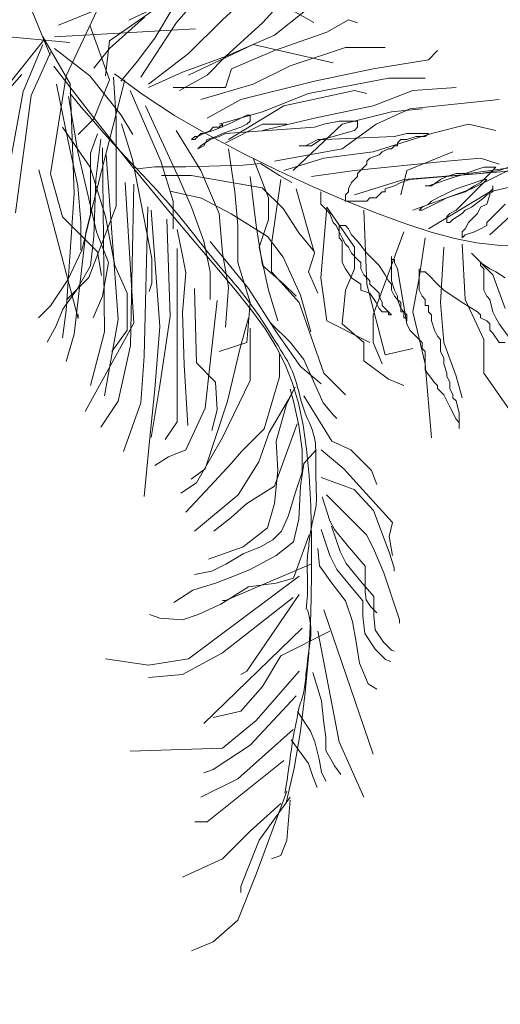
# Model space of a CAD drawing. Units: millimetres. Extents: x 595116 to 630915, y 909473 to 920225.
# Tile 35 of 134: x 629667.505 to 629671.98, y 919163.952 to 919173.119. Entities that reach past the tile are written whole.
import ezdxf

# ---------------------------------------------------------------- set-up
doc = ezdxf.new("R2010")
doc.units = ezdxf.units.MM
doc.layers.add('Dimension', color=3, linetype='Continuous', lineweight=18)
doc.layers.add('L-PLNT', color=85, linetype='Continuous', lineweight=13)
doc.styles.get("Standard").update_dxf_attribs({"font": 'arial.ttf'})
doc.dimstyles.new('ISO-25', dxfattribs={"dimtxt": 9, "dimasz": 6, "dimexe": 1.25, "dimexo": 0.625, "dimtad": 1, "dimlunit": 4, "dimtxsty": 'Standard', "dimcen": 2.5, "dimadec": 0, "dimazin": 0, "dimtfac": 1, "dimtmove": 0, "dimatfit": 3, "dimfxl": 1, "dimarcsym": 0})

# ---------------------------------------------------------------- blocks, each defined once
blk = doc.blocks.new('A$C4FB75ABC')
for p, q in [((2.6324, 2.4053), (2.7073, 2.2214)), ((3.0207, 2.3031), (3.1093, 2.4053)), ((3.1344, 2.3096), (3.2259, 2.3934)), ((3.2335, 2.302), (3.3174, 2.3934)), ((2.7277, 2.2964), (2.8733, 2.3546)), ((2.8539, 2.2576), (2.9801, 2.3449)), ((2.9022, 2.3089), (3.0036, 2.3566)), ((2.8248, 2.3352), (2.7471, 2.1703)), ((2.9666, 2.2638), (3.0123, 2.3401)), ((3.264, 2.2715), (3.3403, 2.3324)), ((3.3079, 2.3327), (3.3615, 2.3029)), ((2.8054, 2.2964), (2.8539, 2.1606)), ((2.8539, 2.2382), (2.9413, 2.3158)), ((2.9321, 2.167), (3.0207, 2.3031)), ((3.0505, 2.2257), (3.1344, 2.3096)), ((3.142, 2.2181), (3.2335, 2.302)), ((3.3937, 2.2791), (3.447, 2.3096)), ((3.447, 2.3096), (3.4699, 2.302)), ((2.7559, 2.2536), (2.4852, 2.2785)), ((2.718, 2.2673), (3.0675, 2.2867)), ((3.142, 2.2181), (3.264, 2.2715)), ((3.264, 2.2334), (3.3937, 2.2791)), ((2.6937, 2.2623), (2.4825, 1.9967)), ((2.6889, 2.2479), (2.6404, 2.1315)), ((2.6889, 2.2673), (2.7568, 2.1509)), ((2.8442, 2.1703), (2.8539, 2.2576)), ((2.9208, 2.2029), (2.9666, 2.2638)), ((3.0505, 2.1724), (3.2106, 2.2486)), ((3.2106, 2.2486), (3.4089, 2.2029)), ((2.7083, 2.2285), (2.6598, 2.1218)), ((2.718, 2.2382), (2.8054, 2.1703)), ((2.8151, 2.1897), (2.8539, 2.2382)), ((2.9513, 2.1495), (3.0505, 2.2257)), ((3.1572, 2.1876), (3.264, 2.2334)), ((3.3021, 2.1952), (3.4394, 2.241)), ((3.4394, 2.241), (3.5385, 2.241)), ((3.6453, 2.2105), (3.6682, 2.2334)), ((2.8827, 2.1571), (2.9208, 2.2029)), ((3.0352, 2.18), (3.142, 2.2181)), ((3.0962, 2.1724), (3.142, 2.2181)), ((3.508, 2.1876), (3.6453, 2.2105)), ((2.6368, 2.1742), (2.4628, 1.9766)), ((2.7162, 2.1941), (2.8268, 2.0511)), ((2.9375, 2.1232), (2.8667, 2.1755)), ((2.9513, 2.1419), (3.0352, 2.18)), ((3.142, 2.1419), (3.1572, 2.1876)), ((3.2106, 2.1495), (3.3021, 2.1952)), ((3.3631, 2.1571), (3.508, 2.1876)), ((2.7471, 2.1703), (2.7083, 1.9277)), ((2.7225, 2.1495), (2.753, 2.0047)), ((2.7568, 2.1509), (2.7666, 1.8792)), ((2.8927, 2.1606), (2.7957, 1.7822)), ((2.8054, 2.1703), (2.883, 2.0733)), ((2.8539, 2.1606), (2.8151, 2.0636)), ((2.864, 2.167), (2.8708, 2.0648)), ((3.0276, 2.1343), (3.0962, 2.1724)), ((3.081, 2.1114), (3.2106, 2.1495)), ((3.1801, 2.1114), (3.3631, 2.1571)), ((3.3479, 2.1266), (3.5462, 2.1648)), ((3.5462, 2.1648), (3.6377, 2.1648)), ((2.6404, 2.1315), (2.5918, 1.8695)), ((2.7555, 2.1274), (2.7844, 2.0931)), ((2.9056, 2.1343), (2.9818, 1.9589)), ((3.0123, 2.1419), (3.142, 2.1419)), ((3.2335, 2.0809), (3.3479, 2.1266)), ((3.2869, 2.0961), (3.4623, 2.1343)), ((3.4623, 2.1343), (3.4928, 2.1266)), ((3.508, 2.0961), (3.6072, 2.1343)), ((3.6072, 2.1343), (3.714, 2.1419)), ((2.6598, 2.1218), (2.6209, 1.8307)), ((2.753, 2.119), (2.7759, 1.9818)), ((3.0158, 2.0725), (2.9375, 2.1232)), ((3.0962, 2.0657), (3.1801, 2.1114)), ((3.5996, 2.0885), (3.8207, 2.1114)), ((2.7844, 2.0931), (2.8104, 2.0628)), ((2.9437, 2.0961), (3.0276, 1.9132)), ((3.1267, 2.0504), (3.2335, 2.0809)), ((3.1496, 2.0123), (3.2869, 2.0961)), ((3.3631, 2.0657), (3.508, 2.0961)), ((3.4318, 2.0504), (3.5538, 2.0809)), ((3.5157, 2.0504), (3.5996, 2.0885)), ((3.5538, 2.0809), (3.6301, 2.0885)), ((2.8151, 2.0636), (2.7763, 2.0248)), ((2.8104, 2.0628), (2.8339, 2.0359)), ((2.8708, 2.0648), (2.8708, 1.8469)), ((2.883, 2.0733), (2.9122, 2.0248)), ((3.0992, 2.0238), (3.0158, 2.0725)), ((3.1649, 2.058), (3.1496, 2.0504)), ((3.1801, 2.0657), (3.1649, 2.058)), ((3.1954, 2.0733), (3.1801, 2.0657)), ((3.203, 2.0733), (3.1954, 2.0733)), ((3.1954, 2.0504), (3.203, 2.058)), ((3.203, 2.058), (3.203, 2.0733)), ((3.2335, 2.0352), (3.3631, 2.0657)), ((3.4242, 2.058), (3.386, 2.0504)), ((3.4699, 2.058), (3.4242, 2.058)), ((3.4699, 2.0428), (3.4699, 2.058)), ((2.7378, 2.0428), (2.8064, 1.9437)), ((2.8268, 2.0511), (2.9214, 1.9326)), ((2.8339, 2.0359), (2.8551, 2.0121)), ((2.8844, 2.0512), (2.9117, 1.9627)), ((3.02, 2.0352), (3.081, 1.9361)), ((3.0734, 2.0199), (3.081, 2.0275)), ((3.0886, 2.0275), (3.0734, 2.0199)), ((3.081, 2.0275), (3.0886, 2.0275)), ((3.1115, 2.0352), (3.0886, 2.0275)), ((3.0886, 2.0275), (3.1039, 2.0352)), ((3.1039, 2.0352), (3.1115, 2.0428)), ((3.1496, 2.0504), (3.1115, 2.0352)), ((3.1115, 2.0428), (3.1267, 2.0428)), ((3.1191, 2.0199), (3.1344, 2.0275)), ((3.1267, 2.0428), (3.1344, 2.0504)), ((3.142, 2.0275), (3.1267, 2.0199)), ((3.1344, 2.0504), (3.1344, 2.0428)), ((3.1344, 2.0275), (3.1801, 2.0428)), ((3.142, 2.0047), (3.2335, 2.0504)), ((3.3631, 2.0428), (3.142, 2.0275)), ((3.1801, 2.0428), (3.1954, 2.0504)), ((3.2335, 2.0504), (3.2945, 2.0504)), ((3.3098, 1.9361), (3.4318, 2.0504)), ((3.386, 2.0504), (3.3631, 2.0428)), ((3.4089, 2.0199), (3.4623, 2.0352)), ((3.4318, 1.9894), (3.5157, 2.0504)), ((3.4623, 2.0352), (3.4699, 2.0428)), ((3.508, 1.9818), (3.6529, 2.0275)), ((3.5919, 2.0275), (3.5614, 2.0199)), ((3.6453, 2.0275), (3.5919, 2.0275)), ((3.6377, 2.0199), (3.6453, 2.0275)), ((3.6529, 2.0275), (3.7445, 2.0504)), ((3.7445, 2.0504), (3.8131, 2.0352)), ((2.753, 2.0047), (2.7759, 1.898)), ((2.8244, 2.0263), (2.8071, 1.979)), ((2.833, 2.0134), (2.8201, 1.9144)), ((2.8551, 2.0121), (2.8744, 1.9909)), ((3.0581, 2.0123), (3.0657, 2.0199)), ((3.0657, 2.0123), (3.0581, 2.0123)), ((3.0734, 2.0199), (3.0657, 2.0123)), ((3.0657, 2.0199), (3.0734, 2.0199)), ((3.1039, 2.0123), (3.081, 1.9971)), ((3.0886, 1.9971), (3.0962, 2.0123)), ((3.0962, 2.0123), (3.1191, 2.0199)), ((3.1858, 1.9776), (3.0992, 2.0238)), ((3.1267, 2.0199), (3.1039, 2.0123)), ((3.3555, 2.0047), (3.3403, 1.9971)), ((3.3708, 2.0123), (3.3555, 2.0047)), ((3.3555, 1.9971), (3.3784, 2.0123)), ((3.386, 2.0123), (3.3708, 2.0123)), ((3.3784, 2.0123), (3.4089, 2.0199)), ((3.5614, 2.0199), (3.386, 2.0123)), ((3.5691, 2.0047), (3.5767, 2.0123)), ((3.5691, 1.9971), (3.5691, 2.0047)), ((3.5767, 2.0123), (3.5919, 2.0123)), ((3.5919, 2.0123), (3.6148, 2.0199)), ((3.6148, 2.0199), (3.6377, 2.0199)), ((2.7759, 1.9818), (2.8217, 1.7836)), ((2.8071, 1.979), (2.8071, 1.9015)), ((2.8373, 1.9919), (2.8416, 1.5357)), ((2.8744, 1.9909), (2.8918, 1.9721)), ((3.081, 1.9971), (3.0734, 1.9894)), ((3.0734, 1.9894), (3.0886, 1.9971)), ((3.1496, 1.9894), (3.1649, 1.8827)), ((3.264, 1.9589), (3.4318, 1.9894)), ((3.3403, 1.9971), (3.325, 1.9971)), ((3.325, 1.9971), (3.3555, 1.9971)), ((3.386, 1.9666), (3.508, 1.9818)), ((3.5233, 1.9742), (3.5309, 1.9818)), ((3.5309, 1.9818), (3.5462, 1.9894)), ((3.5462, 1.9894), (3.5538, 1.9894)), ((3.5538, 1.9894), (3.5614, 1.9971)), ((3.5614, 1.9971), (3.5691, 1.9971)), ((3.5919, 1.9361), (3.7063, 1.9818)), ((2.8459, 1.9747), (2.876, 1.5659)), ((2.8918, 1.9721), (2.9078, 1.955)), ((2.9078, 1.955), (2.9225, 1.9395)), ((2.9117, 1.9627), (2.9458, 1.7856)), ((2.9818, 1.9589), (3.0123, 1.8599)), ((3.2732, 1.9345), (3.1858, 1.9776)), ((3.2106, 1.9666), (3.2488, 1.8675)), ((3.2869, 1.9361), (3.386, 1.9666)), ((3.4623, 1.9361), (3.6911, 1.9589)), ((3.4928, 1.9589), (3.5004, 1.9666)), ((3.4928, 1.9513), (3.4928, 1.9589)), ((3.5004, 1.9666), (3.5233, 1.9742)), ((3.6911, 1.9589), (3.775, 1.9666)), ((3.7521, 1.8903), (3.8894, 1.9589)), ((3.775, 1.9666), (3.8207, 1.9513)), ((2.6792, 1.9375), (2.7763, 1.5688)), ((2.8064, 1.9437), (2.8446, 1.8217)), ((2.9214, 1.9326), (3.0014, 1.8351)), ((2.9225, 1.9395), (2.9361, 1.925)), ((2.9234, 1.9402), (2.9664, 1.9445)), ((2.9664, 1.9445), (3.0439, 1.9445)), ((3.0439, 1.9445), (3.186, 1.9488)), ((3.081, 1.9361), (3.1267, 1.8294)), ((3.186, 1.9488), (3.2291, 1.9531)), ((3.2291, 1.9531), (3.2764, 1.923)), ((3.3593, 1.8951), (3.2732, 1.9345)), ((3.3555, 1.9208), (3.4623, 1.9361)), ((3.4699, 1.9285), (3.4852, 1.9437)), ((3.4852, 1.9437), (3.4928, 1.9513)), ((3.5767, 1.8751), (3.5919, 1.9361)), ((3.5843, 1.9132), (3.8665, 1.9361)), ((3.7826, 1.9437), (3.7368, 1.9285)), ((3.7445, 1.9285), (3.9122, 1.9513)), ((3.8207, 1.9361), (3.775, 1.9285)), ((3.7826, 1.9132), (3.8131, 1.9437)), ((3.8131, 1.9437), (3.7826, 1.9437)), ((3.7978, 1.8827), (4.0495, 1.9437)), ((3.8665, 1.9513), (3.8207, 1.9361)), ((2.7083, 1.9277), (2.7374, 1.821)), ((2.8201, 1.9144), (2.8158, 1.7724)), ((2.8933, 1.9058), (2.9148, 1.5573)), ((2.9361, 1.925), (2.9489, 1.9114)), ((2.9489, 1.9114), (2.9609, 1.8985)), ((2.9837, 1.923), (3.0569, 1.923)), ((3.0276, 1.9132), (3.0581, 1.8446)), ((3.0569, 1.923), (3.2334, 1.8929)), ((3.203, 1.9208), (3.2182, 1.7989)), ((3.2793, 1.9132), (3.2564, 1.7531)), ((3.2764, 1.923), (3.3066, 1.9058)), ((3.447, 1.8903), (3.4547, 1.9056)), ((3.4547, 1.9056), (3.4623, 1.9132)), ((3.4623, 1.9132), (3.4699, 1.9208)), ((3.4623, 1.8751), (3.5843, 1.9132)), ((3.4699, 1.9208), (3.4699, 1.9285)), ((3.5767, 1.9056), (3.5614, 1.898)), ((3.5996, 1.9132), (3.5767, 1.9056)), ((3.775, 1.9285), (3.5996, 1.9132)), ((3.6453, 1.898), (3.714, 1.9208)), ((3.6758, 1.9132), (3.6529, 1.898)), ((3.6911, 1.9208), (3.6758, 1.9132)), ((3.714, 1.9285), (3.6911, 1.9208)), ((3.7368, 1.9285), (3.714, 1.9285)), ((3.714, 1.9208), (3.7445, 1.9285)), ((3.7368, 1.898), (3.7826, 1.9132)), ((3.7597, 1.8827), (3.7826, 1.9056)), ((3.775, 1.9056), (3.7597, 1.898)), ((3.7826, 1.9132), (3.775, 1.9056)), ((3.7826, 1.9056), (3.7902, 1.9132)), ((3.7902, 1.9132), (3.7826, 1.9132)), ((2.7759, 1.898), (2.7836, 1.8065)), ((2.8071, 1.9015), (2.8071, 1.8241)), ((2.9148, 1.9015), (2.9062, 1.5013)), ((2.9609, 1.8985), (2.9724, 1.8861)), ((2.9724, 1.8861), (2.9834, 1.874)), ((3.0052, 1.8843), (3.0827, 1.8671)), ((3.1649, 1.8827), (3.1725, 1.7989)), ((3.2334, 1.8929), (3.285, 1.8413)), ((3.3174, 1.8903), (3.3631, 1.7303)), ((3.4421, 1.8597), (3.3593, 1.8951)), ((3.3784, 1.8827), (3.3784, 1.8522)), ((3.4394, 1.8751), (3.447, 1.8827)), ((3.447, 1.8827), (3.447, 1.8903)), ((3.5309, 1.8827), (3.5233, 1.8751)), ((3.5385, 1.8827), (3.5309, 1.8827)), ((3.5614, 1.898), (3.5385, 1.8903)), ((3.5385, 1.8903), (3.5385, 1.8827)), ((3.6072, 1.837), (3.7521, 1.8903)), ((3.6529, 1.898), (3.6377, 1.898)), ((3.6377, 1.898), (3.6453, 1.898)), ((3.6453, 1.7913), (3.7978, 1.8827)), ((3.6682, 1.8675), (3.714, 1.8903)), ((3.7368, 1.8827), (3.6911, 1.8675)), ((3.714, 1.8903), (3.7368, 1.898)), ((3.7597, 1.898), (3.7368, 1.8827)), ((3.7521, 1.8751), (3.7597, 1.8827)), ((3.8055, 1.8827), (3.7902, 1.8751)), ((3.7978, 1.8827), (3.8055, 1.8903)), ((3.7978, 1.8751), (3.7978, 1.8827)), ((3.8055, 1.8903), (3.8055, 1.898)), ((3.8055, 1.898), (3.8055, 1.8827)), ((2.7666, 1.8792), (2.7471, 1.5882)), ((2.9834, 1.874), (2.994, 1.862)), ((2.994, 1.862), (3.0045, 1.8499)), ((3.0123, 1.8599), (3.0123, 1.7913)), ((3.0827, 1.8671), (3.1559, 1.8284)), ((3.2488, 1.8675), (3.2488, 1.8141)), ((3.4394, 1.8599), (3.4394, 1.8751)), ((3.4928, 1.8599), (3.4394, 1.8599)), ((3.5192, 1.829), (3.4421, 1.8597)), ((3.5004, 1.8675), (3.4928, 1.8599)), ((3.5157, 1.8675), (3.5004, 1.8675)), ((3.5233, 1.8751), (3.5157, 1.8675)), ((3.6453, 1.8522), (3.6529, 1.8599)), ((3.6529, 1.8599), (3.6682, 1.8675)), ((3.6758, 1.8599), (3.6606, 1.8522)), ((3.6911, 1.8675), (3.6758, 1.8599)), ((3.714, 1.837), (3.7368, 1.8599)), ((3.7368, 1.8599), (3.7521, 1.8751)), ((3.7826, 1.8675), (3.7521, 1.8446)), ((3.7902, 1.8751), (3.7826, 1.8675)), ((3.7902, 1.8522), (3.7978, 1.8751)), ((3.7978, 1.776), (3.897, 1.8675)), ((2.8708, 1.8469), (2.8027, 1.6699)), ((2.9492, 1.8456), (2.9406, 1.4755)), ((2.9578, 1.837), (2.9794, 1.5486)), ((3.0014, 1.8351), (3.0686, 1.7552)), ((3.0045, 1.8499), (3.0149, 1.8377)), ((3.0149, 1.8377), (3.0253, 1.8251)), ((3.0581, 1.8446), (3.0886, 1.7608)), ((3.285, 1.8413), (3.3238, 1.781)), ((3.3784, 1.8522), (3.3937, 1.837)), ((3.3937, 1.8446), (3.3784, 1.6693)), ((3.3937, 1.8446), (3.4623, 1.7455)), ((3.3937, 1.837), (3.4013, 1.8294)), ((3.4852, 1.837), (3.4928, 1.6541)), ((3.6224, 1.837), (3.6301, 1.8446)), ((3.6301, 1.837), (3.6224, 1.837)), ((3.6606, 1.8522), (3.6301, 1.837)), ((3.6301, 1.8446), (3.6453, 1.8522)), ((3.6987, 1.8294), (3.714, 1.837)), ((3.7368, 1.837), (3.7292, 1.8294)), ((3.7521, 1.8446), (3.7368, 1.837)), ((3.7673, 1.8294), (3.775, 1.8446)), ((3.775, 1.8446), (3.7902, 1.8522)), ((3.8207, 1.837), (3.8131, 1.8294)), ((3.836, 1.8522), (3.8207, 1.837)), ((2.7374, 1.821), (2.8248, 1.7337)), ((2.8071, 1.8241), (2.7856, 1.738)), ((2.8446, 1.8217), (2.8674, 1.6998)), ((2.9966, 1.8154), (3.0052, 1.5745)), ((3.0253, 1.8251), (3.0358, 1.8122)), ((3.0358, 1.8122), (3.0461, 1.7993)), ((3.1267, 1.8294), (3.1344, 1.7303)), ((3.1559, 1.8284), (3.2463, 1.7724)), ((3.2488, 1.8141), (3.2259, 1.7455)), ((3.4013, 1.8294), (3.4089, 1.8065)), ((3.5892, 1.8034), (3.5192, 1.829)), ((3.6911, 1.8217), (3.6987, 1.8294)), ((3.6911, 1.8065), (3.6911, 1.8217)), ((3.7063, 1.8141), (3.6987, 1.8065)), ((3.7292, 1.8294), (3.7063, 1.8141)), ((3.7445, 1.8065), (3.7673, 1.8294)), ((3.8131, 1.8294), (3.7902, 1.8065)), ((2.7836, 1.8065), (2.7836, 1.7379)), ((2.8217, 1.7836), (2.8522, 1.7074)), ((2.9458, 1.7856), (2.9594, 1.7175)), ((3.0224, 1.7896), (3.0353, 1.7251)), ((3.0461, 1.7993), (3.0562, 1.7866)), ((3.0562, 1.7866), (3.0659, 1.7741)), ((3.1725, 1.7989), (3.1725, 1.7074)), ((3.2182, 1.7989), (3.2335, 1.6998)), ((3.4089, 1.8065), (3.4165, 1.7989)), ((3.4165, 1.7989), (3.4242, 1.7836)), ((3.4242, 1.7684), (3.4242, 1.7989)), ((3.4242, 1.7989), (3.4394, 1.7989)), ((3.4242, 1.7836), (3.4318, 1.7684)), ((3.4394, 1.7989), (3.447, 1.7913)), ((3.447, 1.7913), (3.4547, 1.776)), ((3.5843, 1.7836), (3.508, 1.5778)), ((3.6527, 1.7828), (3.5892, 1.8034)), ((3.7109, 1.7672), (3.6527, 1.7828)), ((3.6987, 1.8065), (3.6911, 1.8065)), ((3.7292, 1.7836), (3.7368, 1.7913)), ((3.7292, 1.7684), (3.7292, 1.7836)), ((3.7368, 1.7913), (3.7445, 1.8065)), ((3.7597, 1.7836), (3.7368, 1.776)), ((3.775, 1.7913), (3.7597, 1.7836)), ((3.7902, 1.7989), (3.775, 1.7913)), ((3.7902, 1.8065), (3.7902, 1.7989)), ((2.7957, 1.7822), (2.7666, 1.53)), ((2.8158, 1.7724), (2.8071, 1.6993)), ((3.0659, 1.7741), (3.0752, 1.7623)), ((3.0752, 1.7623), (3.084, 1.7511)), ((3.0886, 1.7608), (3.1039, 1.6845)), ((3.1042, 1.7595), (3.1989, 1.6433)), ((3.2463, 1.7724), (3.285, 1.7208)), ((3.3238, 1.781), (3.3625, 1.7337)), ((3.4318, 1.7608), (3.4242, 1.7684)), ((3.4318, 1.7684), (3.4394, 1.7531)), ((3.4318, 1.7074), (3.4318, 1.7608)), ((3.4547, 1.776), (3.4699, 1.7608)), ((3.4699, 1.7608), (3.4928, 1.7303)), ((3.6377, 1.7684), (3.6224, 1.6693)), ((3.7651, 1.7564), (3.7109, 1.7672)), ((3.7368, 1.776), (3.7292, 1.7684)), ((2.7856, 1.738), (2.7512, 1.6648)), ((3.0224, 1.7423), (3.0224, 1.312)), ((3.0686, 1.7552), (3.1246, 1.6894)), ((3.084, 1.7511), (3.0921, 1.7408)), ((3.0921, 1.7408), (3.0994, 1.7316)), ((3.2259, 1.7455), (3.2488, 1.6388)), ((3.2564, 1.7531), (3.2564, 1.6845)), ((3.4394, 1.7531), (3.447, 1.7455)), ((3.447, 1.7455), (3.4547, 1.7303)), ((3.4623, 1.7455), (3.4623, 1.6922)), ((3.6834, 1.7455), (3.6758, 1.6083)), ((3.7292, 1.7531), (3.7368, 1.6159)), ((3.8165, 1.7504), (3.7651, 1.7564)), ((3.8664, 1.749), (3.8165, 1.7504)), ((2.8248, 1.7337), (2.8345, 1.6755)), ((2.9594, 1.7175), (2.9594, 1.6563)), ((3.0353, 1.7251), (3.0439, 1.682)), ((3.0994, 1.7316), (3.1062, 1.7232)), ((3.1062, 1.7232), (3.1126, 1.7155)), ((3.1126, 1.7155), (3.1186, 1.7083)), ((3.1344, 1.7303), (3.1496, 1.6464)), ((3.285, 1.7208), (3.3281, 1.6261)), ((3.3631, 1.7303), (3.3479, 1.6845)), ((3.4547, 1.7303), (3.4699, 1.715)), ((3.4699, 1.715), (3.4775, 1.7074)), ((3.4928, 1.7303), (3.508, 1.715)), ((3.508, 1.715), (3.5233, 1.6998)), ((3.5538, 1.7227), (3.5538, 1.715)), ((3.5538, 1.6617), (3.5538, 1.7227)), ((3.5538, 1.715), (3.5614, 1.715)), ((3.5614, 1.715), (3.5614, 1.7074)), ((3.7521, 1.7303), (3.8055, 1.6769)), ((2.8071, 1.6993), (2.7727, 1.639)), ((2.8522, 1.7074), (2.8369, 1.6236)), ((2.8674, 1.6998), (2.8979, 1.6312)), ((3.1186, 1.7083), (3.1246, 1.7013)), ((3.1246, 1.7013), (3.1305, 1.6944)), ((3.1246, 1.6894), (3.1709, 1.6342)), ((3.1305, 1.6944), (3.1367, 1.6873)), ((3.1367, 1.6873), (3.1432, 1.6798)), ((3.1725, 1.7074), (3.203, 1.6083)), ((3.2335, 1.6998), (3.2869, 1.6541)), ((3.4394, 1.6922), (3.4318, 1.7074)), ((3.4547, 1.6693), (3.4394, 1.6922)), ((3.4623, 1.6922), (3.4394, 1.6388)), ((3.4775, 1.7074), (3.4775, 1.6922)), ((3.4775, 1.6922), (3.4852, 1.6769)), ((3.5233, 1.6998), (3.5385, 1.6769)), ((3.5614, 1.7074), (3.5691, 1.6922)), ((3.5691, 1.6922), (3.5919, 1.555)), ((3.6224, 1.6922), (3.6224, 1.6845)), ((3.6224, 1.6388), (3.6224, 1.6922)), ((3.775, 1.6998), (3.775, 1.7074)), ((3.775, 1.7074), (3.7978, 1.6922)), ((3.7826, 1.6922), (3.775, 1.6998)), ((3.7826, 1.6388), (3.7826, 1.6922)), ((3.7978, 1.6922), (3.8131, 1.6845)), ((2.7512, 1.6648), (2.7081, 1.6003)), ((2.8027, 1.6699), (2.7482, 1.6154)), ((3.0439, 1.682), (3.0353, 1.5831)), ((3.1039, 1.6845), (3.1039, 1.6159)), ((3.1432, 1.6798), (3.1502, 1.6718)), ((3.1502, 1.6718), (3.1576, 1.6632)), ((3.1576, 1.6632), (3.1654, 1.654)), ((3.2564, 1.6845), (3.325, 1.6083)), ((3.3479, 1.6845), (3.3708, 1.6312)), ((3.3784, 1.6693), (3.3937, 1.5626)), ((3.4775, 1.6541), (3.4547, 1.6693)), ((3.4852, 1.6769), (3.4928, 1.6693)), ((3.4928, 1.6693), (3.5004, 1.6617)), ((3.5004, 1.6617), (3.5004, 1.6541)), ((3.5385, 1.6769), (3.5462, 1.6617)), ((3.5462, 1.6617), (3.5538, 1.6541)), ((3.5614, 1.6388), (3.5538, 1.6617)), ((3.6224, 1.6693), (3.6072, 1.5855)), ((3.6224, 1.6845), (3.6377, 1.6845)), ((3.6377, 1.6845), (3.6453, 1.6769)), ((3.6453, 1.6769), (3.6682, 1.6541)), ((3.8055, 1.6769), (3.836, 1.5931)), ((3.8131, 1.6845), (3.836, 1.6693)), ((2.7727, 1.639), (2.7383, 1.5917)), ((2.9594, 1.6563), (2.9526, 1.6358)), ((3.0655, 1.6433), (3.0698, 1.4583)), ((3.1496, 1.6464), (3.142, 1.5473)), ((3.1654, 1.654), (3.1735, 1.6443)), ((3.1735, 1.6443), (3.1819, 1.634)), ((3.1989, 1.6433), (3.2678, 1.5357)), ((3.2488, 1.6388), (3.2716, 1.5626)), ((3.2869, 1.6541), (3.3174, 1.6236)), ((3.4394, 1.6388), (3.4318, 1.555)), ((3.4775, 1.6388), (3.4775, 1.6541)), ((3.5004, 1.6312), (3.4775, 1.6388)), ((3.4928, 1.6541), (3.5385, 1.4787)), ((3.5004, 1.6541), (3.5157, 1.6388)), ((3.5157, 1.6388), (3.5233, 1.6312)), ((3.5538, 1.6541), (3.5538, 1.6388)), ((3.5538, 1.6388), (3.5614, 1.6236)), ((3.5691, 1.6236), (3.5614, 1.6388)), ((3.6301, 1.6236), (3.6224, 1.6388)), ((3.6682, 1.6541), (3.6834, 1.6388)), ((3.6834, 1.6388), (3.7292, 1.6083)), ((3.7902, 1.6236), (3.7826, 1.6388)), ((2.8369, 1.6236), (2.8141, 1.5702)), ((2.8979, 1.6312), (2.8979, 1.5397)), ((3.1214, 1.6132), (3.1042, 1.4583)), ((3.1709, 1.6342), (3.2091, 1.5863)), ((3.1819, 1.634), (3.1904, 1.6232)), ((3.1904, 1.6232), (3.1991, 1.6119)), ((3.1991, 1.6119), (3.2078, 1.6)), ((3.3281, 1.6261), (3.3539, 1.5357)), ((3.5157, 1.6083), (3.5004, 1.6312)), ((3.5233, 1.6312), (3.5233, 1.6236)), ((3.5233, 1.6236), (3.5309, 1.6083)), ((3.5614, 1.6236), (3.5691, 1.6159)), ((3.5691, 1.6159), (3.5691, 1.6236)), ((3.5691, 1.6159), (3.5767, 1.6083)), ((3.5767, 1.5931), (3.5691, 1.6159)), ((3.6377, 1.6159), (3.6301, 1.6236)), ((3.6377, 1.6007), (3.6377, 1.6159)), ((3.7368, 1.6159), (3.7826, 1.5168)), ((3.7978, 1.6159), (3.7902, 1.6236)), ((3.8055, 1.5855), (3.7978, 1.6159)), ((2.7081, 1.6003), (2.678, 1.5702)), ((2.7383, 1.5917), (2.721, 1.5486)), ((2.7471, 1.5882), (2.7374, 1.5203)), ((3.203, 1.6083), (3.1954, 1.5092)), ((3.2078, 1.6), (3.2166, 1.5877)), ((3.2166, 1.5877), (3.2252, 1.575)), ((3.325, 1.6083), (3.386, 1.433)), ((3.5233, 1.5931), (3.5157, 1.6083)), ((3.5309, 1.5855), (3.5233, 1.5931)), ((3.5309, 1.6083), (3.5309, 1.6007)), ((3.5309, 1.6007), (3.5385, 1.5931)), ((3.5385, 1.5931), (3.5462, 1.5855)), ((3.5767, 1.6083), (3.5767, 1.5855)), ((3.5843, 1.5855), (3.5767, 1.5931)), ((3.6453, 1.6007), (3.6377, 1.6007)), ((3.6453, 1.5855), (3.6453, 1.6007)), ((3.6758, 1.6083), (3.6834, 1.5092)), ((3.7292, 1.6083), (3.7673, 1.5855)), ((2.7763, 1.5688), (2.7763, 1.5785)), ((2.876, 1.5659), (2.8416, 1.3765)), ((3.0052, 1.5745), (2.9794, 1.4023)), ((3.0353, 1.5831), (3.0396, 1.454)), ((3.1989, 1.5702), (3.1774, 1.4927)), ((3.2091, 1.5863), (3.241, 1.5422)), ((3.2252, 1.575), (3.2338, 1.5622)), ((3.508, 1.5778), (3.508, 1.5092)), ((3.5462, 1.5855), (3.5309, 1.5855)), ((3.5462, 1.5855), (3.5462, 1.5778)), ((3.5538, 1.5778), (3.5462, 1.5855)), ((3.5462, 1.5778), (3.5538, 1.5778)), ((3.5767, 1.5855), (3.5843, 1.5855)), ((3.5843, 1.5855), (3.5843, 1.5702)), ((3.5919, 1.5778), (3.5843, 1.5855)), ((3.5843, 1.5702), (3.5919, 1.5702)), ((3.5919, 1.5626), (3.5919, 1.5778)), ((3.5919, 1.5702), (3.5919, 1.5626)), ((3.6072, 1.5855), (3.6377, 1.4559)), ((3.6529, 1.5778), (3.6453, 1.5855)), ((3.6529, 1.5626), (3.6529, 1.5778)), ((3.7673, 1.5855), (3.775, 1.5778)), ((3.775, 1.5778), (3.775, 1.5702)), ((3.775, 1.5702), (3.7902, 1.5626)), ((3.8131, 1.5702), (3.8055, 1.5855)), ((3.8207, 1.555), (3.8131, 1.5702)), ((2.721, 1.5486), (2.6995, 1.5099)), ((2.9148, 1.5573), (2.7942, 1.3378)), ((2.8979, 1.5397), (2.8598, 1.4864)), ((2.9794, 1.5486), (2.9664, 1.3937)), ((3.2032, 1.5443), (3.2032, 1.4152)), ((3.2338, 1.5622), (3.2421, 1.5493)), ((3.241, 1.5422), (3.2678, 1.4987)), ((3.2421, 1.5493), (3.2503, 1.5367)), ((3.2549, 1.5573), (3.3023, 1.5099)), ((3.3937, 1.5626), (3.4852, 1.5168)), ((3.4318, 1.555), (3.4852, 1.5092)), ((3.5919, 1.555), (3.5996, 1.5397)), ((3.5996, 1.5397), (3.6301, 1.5092)), ((3.6606, 1.5397), (3.6529, 1.5626)), ((3.6682, 1.5245), (3.6606, 1.5397)), ((3.7902, 1.5626), (3.7978, 1.555)), ((3.7978, 1.555), (3.7978, 1.5397)), ((3.7978, 1.5397), (3.8055, 1.5321)), ((3.8436, 1.5245), (3.8207, 1.555)), ((2.7666, 1.53), (2.7471, 1.462)), ((2.8416, 1.5357), (2.8071, 1.4023)), ((3.2503, 1.5367), (3.258, 1.5243)), ((3.258, 1.5243), (3.2655, 1.5125)), ((3.2678, 1.5357), (3.3281, 1.4497)), ((3.4852, 1.5168), (3.5004, 1.5092)), ((3.6758, 1.5168), (3.6682, 1.5245)), ((3.6758, 1.4864), (3.6758, 1.5168)), ((3.7826, 1.5168), (3.7826, 1.433)), ((3.8055, 1.5321), (3.8207, 1.5092)), ((2.9062, 1.5013), (2.876, 1.3636)), ((3.1954, 1.5092), (3.1267, 1.4864)), ((3.1774, 1.4927), (3.1473, 1.3636)), ((3.2655, 1.5125), (3.2724, 1.5013)), ((3.2678, 1.4987), (3.2902, 1.4543)), ((3.2724, 1.5013), (3.2789, 1.491)), ((3.2789, 1.491), (3.2849, 1.4813)), ((3.3023, 1.5099), (3.3367, 1.4669)), ((3.4852, 1.5092), (3.4852, 1.4635)), ((3.508, 1.5092), (3.5309, 1.4559)), ((3.5385, 1.4787), (3.6072, 1.494)), ((3.6301, 1.5092), (3.6301, 1.494)), ((3.6301, 1.494), (3.6377, 1.4864)), ((3.6834, 1.5092), (3.714, 1.4254)), ((3.8207, 1.5092), (3.836, 1.5092)), ((2.9406, 1.4755), (2.932, 1.3593)), ((3.2764, 1.4798), (3.2764, 1.4239)), ((3.2849, 1.4813), (3.2904, 1.4721)), ((3.2904, 1.4721), (3.2955, 1.4632)), ((3.3367, 1.4669), (3.3841, 1.3593)), ((3.6377, 1.4864), (3.6377, 1.4406)), ((3.6834, 1.4711), (3.6758, 1.4864)), ((3.6834, 1.4559), (3.6834, 1.4711)), ((3.0396, 1.454), (3.0483, 1.3034)), ((3.0698, 1.4583), (3.1171, 1.4109)), ((3.1042, 1.4583), (3.0913, 1.3464)), ((3.2902, 1.4543), (3.3086, 1.4079)), ((3.2955, 1.4632), (3.3002, 1.4545)), ((3.3002, 1.4545), (3.3045, 1.4458)), ((3.3045, 1.4458), (3.3084, 1.437)), ((3.3281, 1.4497), (3.3798, 1.4066)), ((3.4852, 1.4635), (3.5462, 1.4178)), ((3.6377, 1.4559), (3.6529, 1.2729)), ((3.6911, 1.433), (3.6834, 1.4559)), ((3.2764, 1.4239), (3.2377, 1.2948)), ((3.3084, 1.437), (3.3119, 1.4278)), ((3.3119, 1.4278), (3.3151, 1.4181)), ((3.3151, 1.4181), (3.3181, 1.4081)), ((3.386, 1.433), (3.4394, 1.3796)), ((3.5462, 1.4178), (3.5843, 1.4025)), ((3.6377, 1.4406), (3.6606, 1.4101)), ((3.6911, 1.4254), (3.6911, 1.433)), ((3.6987, 1.4101), (3.6911, 1.4254)), ((3.714, 1.4254), (3.7292, 1.372)), ((3.7826, 1.433), (3.8741, 1.3034)), ((2.9664, 1.3937), (2.9535, 1.2646)), ((2.9794, 1.4023), (2.9578, 1.2732)), ((3.1171, 1.4109), (3.1214, 1.3421)), ((3.2032, 1.4152), (3.1344, 1.2732)), ((3.2937, 1.355), (3.3152, 1.398)), ((3.298, 1.3679), (3.3152, 1.398)), ((3.3023, 1.3937), (3.3109, 1.3636)), ((3.3086, 1.4079), (3.3233, 1.3583)), ((3.3181, 1.4081), (3.3209, 1.3978)), ((3.3209, 1.3978), (3.3236, 1.3873)), ((3.6606, 1.4101), (3.6682, 1.4025)), ((3.6682, 1.4025), (3.6682, 1.3949)), ((3.6682, 1.3949), (3.6834, 1.3796)), ((3.6987, 1.3949), (3.6987, 1.4101)), ((3.7063, 1.3796), (3.6987, 1.3949)), ((3.2506, 1.2861), (3.298, 1.3679)), ((3.3236, 1.3873), (3.3263, 1.3768)), ((3.3263, 1.3768), (3.3291, 1.3664)), ((3.3367, 1.3765), (3.4056, 1.2646)), ((3.6834, 1.3796), (3.6987, 1.3492)), ((3.7063, 1.372), (3.7063, 1.3796)), ((3.714, 1.3644), (3.7063, 1.372)), ((2.876, 1.3636), (2.833, 1.2991)), ((2.932, 1.3593), (2.889, 1.2388)), ((3.0913, 1.3464), (3.0439, 1.2431)), ((3.1473, 1.3636), (3.0913, 1.1958)), ((3.2678, 1.2646), (3.2937, 1.355)), ((3.3109, 1.3636), (3.3238, 1.3034)), ((3.3233, 1.3583), (3.3348, 1.3042)), ((3.3291, 1.3664), (3.332, 1.3561)), ((3.332, 1.3561), (3.3352, 1.3462)), ((3.3352, 1.3462), (3.3388, 1.3366)), ((3.3841, 1.3593), (3.4099, 1.3292)), ((3.6987, 1.3492), (3.714, 1.3187)), ((3.7216, 1.3339), (3.714, 1.3644)), ((3.1214, 1.3421), (3.1085, 1.2905)), ((3.3388, 1.3366), (3.3425, 1.3274)), ((3.3425, 1.3274), (3.3463, 1.3185)), ((3.4099, 1.3292), (3.4185, 1.3206)), ((3.7216, 1.2958), (3.7216, 1.3339)), ((3.0224, 1.312), (2.9923, 1.2689)), ((3.2377, 1.2948), (3.1817, 1.2388)), ((3.3195, 1.3077), (3.2635, 1.1527)), ((3.3238, 1.3034), (3.3324, 1.2431)), ((3.3348, 1.3042), (3.3434, 1.2446)), ((3.3463, 1.3185), (3.3501, 1.3098)), ((3.3501, 1.3098), (3.3537, 1.3013)), ((3.3537, 1.3013), (3.357, 1.2929)), ((3.714, 1.3187), (3.7216, 1.311)), ((3.7216, 1.311), (3.7216, 1.2958)), ((3.1344, 1.2732), (3.0698, 1.1614)), ((3.2248, 1.213), (3.2506, 1.2861)), ((3.357, 1.2929), (3.3598, 1.2846)), ((3.3598, 1.2846), (3.3622, 1.2762)), ((3.3622, 1.2762), (3.3639, 1.2677)), ((2.9535, 1.2646), (2.9406, 1.1269)), ((3.2721, 1.1915), (3.2678, 1.2646)), ((3.3639, 1.2677), (3.365, 1.2592)), ((3.365, 1.2592), (3.3657, 1.2504)), ((3.3657, 1.2504), (3.366, 1.2415)), ((3.4056, 1.2646), (3.453, 1.2431)), ((3.0009, 1.2259), (2.9664, 1.2044)), ((3.0439, 1.2431), (3.0009, 1.2259)), ((3.1817, 1.2388), (3.1559, 1.2087)), ((3.3324, 1.2431), (3.3324, 1.1872)), ((3.3367, 1.2087), (3.3669, 1.2431)), ((3.3434, 1.2446), (3.3495, 1.1781)), ((3.366, 1.2227), (3.3658, 1.2129)), ((3.366, 1.2415), (3.366, 1.2322)), ((3.366, 1.2322), (3.366, 1.2227)), ((3.3798, 1.2431), (3.4357, 1.1958)), ((3.453, 1.2431), (3.5046, 1.1915)), ((3.1559, 1.2087), (3.1042, 1.1527)), ((3.1731, 1.1312), (3.2248, 1.213)), ((3.3281, 1.1527), (3.3367, 1.2087)), ((3.3658, 1.2129), (3.3658, 1.2027)), ((3.3658, 1.2027), (3.3658, 1.1921)), ((3.0913, 1.1958), (3.0569, 1.17)), ((3.2635, 1.1097), (3.2721, 1.1915)), ((3.3324, 1.1872), (3.3152, 1.1355)), ((3.3495, 1.1781), (3.3535, 1.1037)), ((3.3658, 1.1921), (3.366, 1.1812)), ((3.366, 1.1812), (3.3663, 1.1704)), ((3.3798, 1.1743), (3.4616, 1.1441)), ((3.4357, 1.1958), (3.4745, 1.1527)), ((3.5046, 1.1915), (3.5175, 1.1571)), ((3.0698, 1.1614), (3.031, 1.1355)), ((3.1042, 1.1527), (3.0439, 1.0882)), ((3.2635, 1.1527), (3.1946, 1.1097)), ((3.3238, 1.071), (3.3281, 1.1527)), ((3.3663, 1.1704), (3.3667, 1.1597)), ((3.3667, 1.1597), (3.367, 1.1494)), ((3.367, 1.1494), (3.3673, 1.1397)), ((3.4745, 1.1527), (3.5563, 1.0624)), ((3.0655, 1.0409), (3.1731, 1.1312)), ((3.3152, 1.1355), (3.298, 1.0796)), ((3.3673, 1.1397), (3.3675, 1.1308)), ((3.3675, 1.1308), (3.3676, 1.1228)), ((3.3816, 1.1261), (3.4013, 1.0669)), ((3.3927, 1.1312), (3.44, 1.0839)), ((3.4616, 1.1441), (3.5089, 1.0925)), ((3.1946, 1.1097), (3.1559, 1.0753)), ((3.2463, 1.0495), (3.2635, 1.1097)), ((3.3535, 1.1037), (3.3557, 1.0207)), ((3.3663, 1.1006), (3.3657, 1.0966)), ((3.3668, 1.1051), (3.3663, 1.1006)), ((3.3672, 1.1101), (3.3668, 1.1051)), ((3.3675, 1.116), (3.3672, 1.1101)), ((3.3676, 1.1228), (3.3675, 1.116)), ((3.1559, 1.0753), (3.1128, 1.0409)), ((3.298, 1.0796), (3.2807, 1.0409)), ((3.3609, 1.0765), (3.3598, 1.0717)), ((3.362, 1.081), (3.3609, 1.0765)), ((3.3631, 1.0852), (3.362, 1.081)), ((3.364, 1.0891), (3.3631, 1.0852)), ((3.3649, 1.0928), (3.364, 1.0891)), ((3.3657, 1.0966), (3.3649, 1.0928)), ((3.44, 1.0839), (3.4917, 1.0323)), ((3.5089, 1.0925), (3.5477, 0.9892)), ((3.3109, 1.015), (3.3238, 1.071)), ((3.3551, 1.0505), (3.3541, 1.0448)), ((3.3563, 1.056), (3.3551, 1.0505)), ((3.3574, 1.0614), (3.3563, 1.056)), ((3.3586, 1.0667), (3.3574, 1.0614)), ((3.3598, 1.0717), (3.3586, 1.0667)), ((3.4013, 1.0669), (3.4121, 1.0454)), ((3.4053, 1.0537), (3.4263, 0.991)), ((3.5563, 1.0624), (3.5477, 1.028)), ((3.186, 1.0021), (3.2463, 1.0495)), ((3.2807, 1.0409), (3.2592, 1.0193)), ((3.3496, 1.0323), (3.3109, 0.9247)), ((3.3514, 1.0274), (3.3506, 1.0215)), ((3.3522, 1.0332), (3.3514, 1.0274)), ((3.3531, 1.039), (3.3522, 1.0332)), ((3.3541, 1.0448), (3.3531, 1.039)), ((3.3798, 1.0452), (3.4013, 0.9806)), ((3.4121, 1.0454), (3.4447, 1.0056)), ((3.4917, 1.0323), (3.5089, 0.9978)), ((3.5477, 1.028), (3.5563, 0.9806)), ((3.0999, 0.972), (3.186, 1.0021)), ((3.2291, 1.0021), (3.186, 0.9849)), ((3.2592, 1.0193), (3.2291, 1.0021)), ((3.2678, 0.9806), (3.3109, 1.015)), ((3.3485, 1.0039), (3.3478, 0.9982)), ((3.3492, 1.0097), (3.3485, 1.0039)), ((3.3499, 1.0156), (3.3492, 1.0097)), ((3.3506, 1.0215), (3.3499, 1.0156)), ((3.3557, 1.0207), (3.3558, 0.9307)), ((3.4447, 1.0056), (3.4889, 0.9539)), ((3.186, 0.9849), (3.143, 0.9591)), ((3.2032, 0.9462), (3.2678, 0.9806)), ((3.3459, 0.981), (3.3454, 0.9751)), ((3.3465, 0.9868), (3.3459, 0.981)), ((3.3471, 0.9925), (3.3465, 0.9868)), ((3.3478, 0.9982), (3.3471, 0.9925)), ((3.3712, 0.9978), (3.3755, 0.9548)), ((3.4013, 0.9806), (3.4185, 0.9462)), ((3.4263, 0.991), (3.4413, 0.9609)), ((3.5089, 0.9978), (3.5348, 0.9376)), ((3.5477, 0.9892), (3.5606, 0.9505)), ((3.143, 0.9591), (3.1085, 0.9419)), ((3.3555, 0.9604), (3.142, 0.8689)), ((3.3447, 0.9623), (3.3446, 0.9554)), ((3.3446, 0.9554), (3.3447, 0.9479)), ((3.345, 0.9689), (3.3447, 0.9623)), ((3.3454, 0.9751), (3.345, 0.9689)), ((3.3755, 0.9548), (3.4056, 0.9118)), ((3.4413, 0.9609), (3.4779, 0.9162)), ((3.4889, 0.9539), (3.4889, 0.8899)), ((3.325, 0.9299), (3.0505, 0.7241)), ((3.1085, 0.9419), (3.0655, 0.9333)), ((3.1171, 0.9118), (3.1602, 0.929)), ((3.1602, 0.929), (3.2032, 0.9462)), ((3.3447, 0.9479), (3.3449, 0.9399)), ((3.3449, 0.9399), (3.3453, 0.931)), ((3.3453, 0.931), (3.3456, 0.921)), ((3.3558, 0.9307), (3.3535, 0.836)), ((3.4185, 0.9462), (3.4573, 0.8989)), ((3.5348, 0.9376), (3.5735, 0.8214)), ((3.5606, 0.9505), (3.5606, 0.9419)), ((3.0612, 0.8946), (3.1171, 0.9118)), ((3.2678, 0.9118), (3.1989, 0.9032)), ((3.3109, 0.9247), (3.2678, 0.9118)), ((3.3456, 0.921), (3.3457, 0.9097)), ((3.3457, 0.9097), (3.3456, 0.8969)), ((3.4056, 0.9118), (3.44, 0.8687)), ((3.4779, 0.9162), (3.5101, 0.8787)), ((3.0138, 0.8644), (3.0612, 0.8946)), ((3.1989, 0.9032), (3.1301, 0.8601)), ((3.325, 0.8842), (3.1954, 0.6936)), ((3.3451, 0.8822), (3.3441, 0.8655)), ((3.3456, 0.8969), (3.3451, 0.8822)), ((3.4573, 0.8989), (3.4831, 0.8687)), ((3.4889, 0.8899), (3.4909, 0.8704)), ((3.1301, 0.8601), (3.0741, 0.8343)), ((3.3098, 0.8766), (3.1344, 0.7394)), ((3.142, 0.8689), (3.1344, 0.8689)), ((3.3441, 0.8655), (3.3424, 0.8466)), ((3.44, 0.8687), (3.4573, 0.8171)), ((3.4831, 0.8687), (3.4831, 0.83)), ((3.4909, 0.8704), (3.5015, 0.8546)), ((3.5101, 0.8787), (3.5101, 0.8314)), ((2.9794, 0.8257), (2.9535, 0.8343)), ((3.0741, 0.8343), (3.0353, 0.8214)), ((3.3453, 0.8472), (3.3494, 0.8306)), ((3.3535, 0.836), (3.3484, 0.7387)), ((3.3494, 0.8306), (3.3521, 0.8161)), ((3.386, 0.8461), (3.508, 0.4878)), ((3.5015, 0.8546), (3.5172, 0.8388)), ((3.5101, 0.8314), (3.5136, 0.7963)), ((3.0353, 0.8214), (2.9794, 0.8257)), ((3.3521, 0.8161), (3.3535, 0.8034)), ((3.4573, 0.8171), (3.4659, 0.7655)), ((3.4831, 0.83), (3.4874, 0.787)), ((3.5735, 0.8214), (3.5735, 0.8128)), ((3.3326, 0.8003), (3.0886, 0.5641)), ((3.4013, 0.7927), (3.2793, 0.7317)), ((3.3537, 0.7819), (3.3529, 0.7725)), ((3.3535, 0.8034), (3.354, 0.7921)), ((3.354, 0.7921), (3.3537, 0.7819)), ((3.3708, 0.7927), (3.4242, 0.5183)), ((3.4874, 0.787), (3.5132, 0.7482)), ((3.5136, 0.7963), (3.5342, 0.7654)), ((3.3517, 0.7635), (3.3503, 0.7547)), ((3.3529, 0.7725), (3.3517, 0.7635)), ((3.4659, 0.7655), (3.4745, 0.7138)), ((3.5342, 0.7654), (3.5536, 0.746)), ((3.1344, 0.7394), (3.0352, 0.686)), ((3.3484, 0.7387), (3.34, 0.641)), ((3.3478, 0.7367), (3.3466, 0.7276)), ((3.349, 0.7457), (3.3478, 0.7367)), ((3.3503, 0.7547), (3.349, 0.7457)), ((3.5132, 0.7482), (3.5391, 0.7224)), ((3.5536, 0.746), (3.5605, 0.7437)), ((2.9513, 0.7089), (2.8446, 0.7241)), ((3.0505, 0.7241), (2.9513, 0.7089)), ((3.2793, 0.7317), (3.2335, 0.6555)), ((3.3445, 0.7097), (3.3435, 0.7011)), ((3.3455, 0.7186), (3.3445, 0.7097)), ((3.3466, 0.7276), (3.3455, 0.7186)), ((3.4745, 0.7138), (3.496, 0.6622)), ((3.5391, 0.7224), (3.552, 0.7181)), ((3.0352, 0.686), (2.9513, 0.6784)), ((3.1954, 0.6936), (3.1801, 0.686)), ((3.325, 0.6936), (3.2182, 0.5717)), ((3.3417, 0.6851), (3.341, 0.6779)), ((3.3426, 0.6929), (3.3417, 0.6851)), ((3.3435, 0.7011), (3.3426, 0.6929)), ((3.3586, 0.6905), (3.3801, 0.6206)), ((3.3395, 0.6648), (3.3388, 0.6589)), ((3.3402, 0.6711), (3.3395, 0.6648)), ((3.341, 0.6779), (3.3402, 0.6711)), ((3.496, 0.6622), (3.5175, 0.6493)), ((3.2335, 0.6555), (3.1801, 0.5945)), ((3.34, 0.641), (3.3282, 0.5451)), ((3.3353, 0.6385), (3.3341, 0.634)), ((3.3363, 0.6432), (3.3353, 0.6385)), ((3.3372, 0.6481), (3.3363, 0.6432)), ((3.338, 0.6533), (3.3372, 0.6481)), ((3.3388, 0.6589), (3.338, 0.6533)), ((3.3174, 0.6327), (3.203, 0.5107)), ((3.3276, 0.6135), (3.3264, 0.6095)), ((3.3289, 0.6175), (3.3276, 0.6135)), ((3.3303, 0.6215), (3.3289, 0.6175)), ((3.3316, 0.6256), (3.3303, 0.6215)), ((3.3329, 0.6297), (3.3316, 0.6256)), ((3.3341, 0.634), (3.3329, 0.6297)), ((3.3801, 0.6206), (3.3855, 0.5721)), ((3.1801, 0.5945), (3.1115, 0.5793)), ((3.3216, 0.5886), (3.3208, 0.584)), ((3.3209, 0.5936), (3.3532, 0.5452)), ((3.3225, 0.593), (3.3216, 0.5886)), ((3.3233, 0.5973), (3.3225, 0.593)), ((3.3242, 0.6014), (3.3233, 0.5973)), ((3.3252, 0.6055), (3.3242, 0.6014)), ((3.3264, 0.6095), (3.3252, 0.6055)), ((3.2182, 0.5717), (3.1344, 0.5031)), ((3.3169, 0.5634), (3.3156, 0.5574)), ((3.3181, 0.5689), (3.3169, 0.5634)), ((3.3191, 0.5742), (3.3181, 0.5689)), ((3.32, 0.5792), (3.3191, 0.5742)), ((3.3208, 0.584), (3.32, 0.5792)), ((3.3855, 0.5721), (3.3909, 0.5291)), ((3.3098, 0.5488), (3.1725, 0.4269)), ((3.3127, 0.5432), (3.3111, 0.5347)), ((3.3282, 0.5451), (3.3124, 0.4531)), ((3.3142, 0.5507), (3.3127, 0.5432)), ((3.3156, 0.5574), (3.3142, 0.5507)), ((3.3532, 0.5452), (3.364, 0.5183)), ((3.3047, 0.5237), (3.3478, 0.4645)), ((3.3075, 0.5137), (3.3055, 0.5008)), ((3.3093, 0.5249), (3.3075, 0.5137)), ((3.3111, 0.5347), (3.3093, 0.5249)), ((3.364, 0.5183), (3.3747, 0.4753)), ((3.3909, 0.5291), (3.3909, 0.4968)), ((3.4242, 0.5183), (3.4852, 0.3811)), ((3.1344, 0.5031), (2.9056, 0.4955)), ((3.203, 0.5107), (3.1115, 0.4497)), ((3.3055, 0.5008), (3.3034, 0.4863)), ((3.3909, 0.4968), (3.407, 0.4699)), ((3.2869, 0.4726), (3.0962, 0.3201)), ((3.3013, 0.4707), (3.2992, 0.4546)), ((3.3034, 0.4863), (3.3013, 0.4707)), ((3.3478, 0.4645), (3.3586, 0.4322)), ((3.3747, 0.4753), (3.3801, 0.443)), ((3.407, 0.4699), (3.4124, 0.4591)), ((3.1115, 0.4497), (3.0886, 0.4421)), ((3.3124, 0.4531), (3.2923, 0.3674)), ((3.2992, 0.4546), (3.297, 0.4387)), ((3.3801, 0.443), (3.3909, 0.4214)), ((3.4124, 0.4591), (3.4286, 0.4376)), ((3.1725, 0.4269), (3.081, 0.3811)), ((3.2949, 0.4237), (3.2929, 0.4103)), ((3.297, 0.4387), (3.2949, 0.4237)), ((3.3586, 0.4322), (3.3693, 0.4053)), ((3.2945, 0.3964), (3.2182, 0.1906)), ((3.2911, 0.3992), (3.2894, 0.3911)), ((3.2929, 0.4103), (3.2911, 0.3992)), ((3.3021, 0.3811), (3.2259, 0.2744)), ((3.3021, 0.3735), (3.2945, 0.2744)), ((3.2793, 0.3659), (3.203, 0.2973)), ((3.0962, 0.3201), (3.0657, 0.3201)), ((3.203, 0.2973), (3.1344, 0.2287)), ((3.2259, 0.2744), (3.1954, 0.1982)), ((3.2945, 0.2744), (3.2793, 0.2363)), ((3.1344, 0.2287), (3.0352, 0.1829)), ((3.2793, 0.2363), (3.2564, 0.2287)), ((3.1954, 0.1982), (3.1801, 0.1601)), ((3.2182, 0.1906), (3.1725, 0.0762)), ((3.1801, 0.1601), (3.1801, 0.1448)), ((3.1725, 0.0762), (3.1115, 0.0229)), ((3.1115, 0.0229), (3.0581, 0))]:
    blk.add_line(p, q)
blk = doc.blocks.new('*D216')
at = {"layer": 'Defpoints', "color": 0, "transparency": 16777216}
for p in [(629743.5408, 919411.9276), (629505.0408, 919411.8279), (629743.5408, 918832.3776)]:
    blk.add_point(p, dxfattribs=at)
at = {"layer": 'Dimension', "color": 0, "lineweight": -2, "transparency": 16777216}
for p, q in [((629743.5408, 919411.3026), (629743.5408, 918831.1276)), ((629505.0408, 919411.2029), (629505.0408, 918831.1276)), ((629511.0408, 918832.3776), (629737.5408, 918832.3776))]:
    blk.add_line(p, q, dxfattribs=at)
at = {"layer": 'Dimension', "color": 0, "transparency": 16777216}
for points in [[(629511.0408, 918833.3776), (629511.0408, 918831.3776), (629505.0408, 918832.3776)], [(629737.5408, 918833.3776), (629737.5408, 918831.3776), (629743.5408, 918832.3776)]]:
    blk.add_solid(points, dxfattribs=at)
at = {"layer": 'Dimension', "color": 0, "transparency": 16777216, "insert": (629624.2908, 918837.656), "char_height": 9, "attachment_point": 5}
blk.add_mtext('19\'-10 1/2"', dxfattribs=at)

msp = doc.modelspace()

# ---------------------------------------------------------------- block references
at = {"layer": 'L-PLNT', "xscale": 3.753413438031968, "yscale": 3.753413438031968, "zscale": 3.753413438031968}
msp.add_blockref('A$C4FB75ABC', (629657.6275, 919164.4492), dxfattribs=at)

# ---------------------------------------------------------------- dimensions: what is measured, and where the dimension line sits
at = {"layer": 'Dimension'}
dim = msp.add_linear_dim(base=(629743.5408, 918832.3776), p1=(629505.0408, 919411.8279), p2=(629743.5408, 919411.9276), dimstyle='ISO-25', override={"dimdec": 1, "dimlfac": 1, "dimrnd": 0, "dimzin": 1, "dimdsep": 46, "dimlunit": 4, "dimfrac": 2}, dxfattribs=at)
dim.commit()
dim.dimension.update_dxf_attribs({"geometry": '*D216', "text_midpoint": (629624.2908, 918837.656)})

doc.saveas('drawing.dxf')
